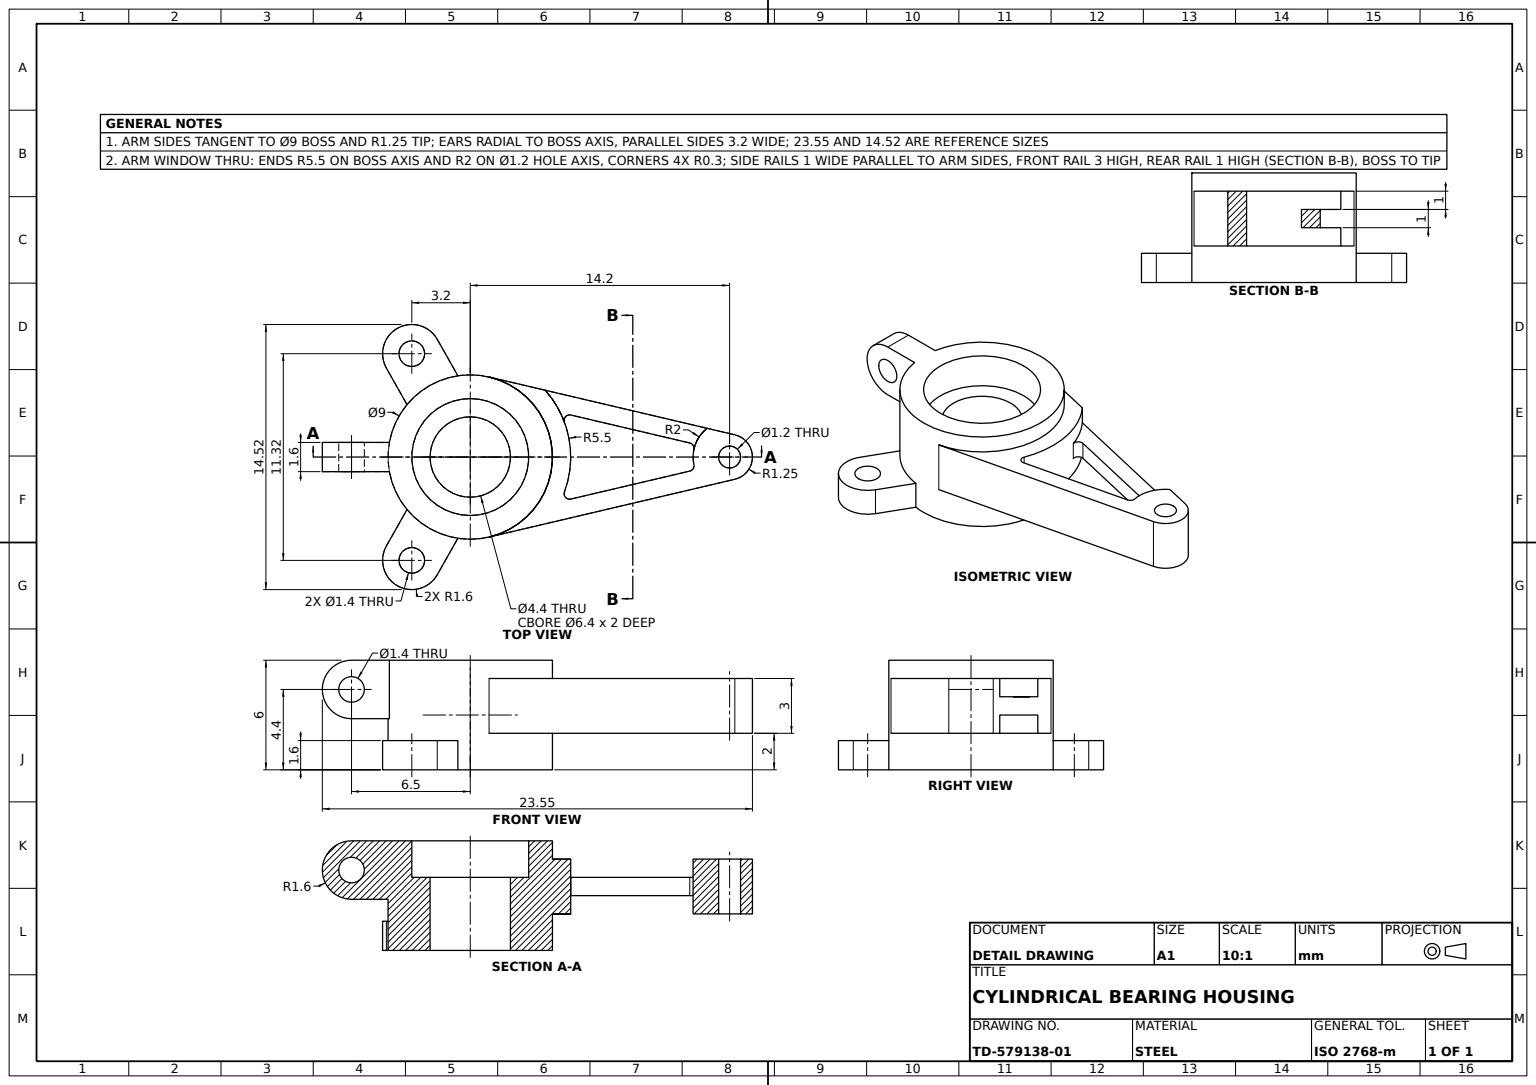
from build123d import *

# Parameters (mm, degrees)
HUB_PROFILE_SKETCH_R           = 4.5
HUB_CYLINDER_DEPTH             = 6
ARM_START                      = -4
ARM_DEPTH                      = 3
FLAT_EAR_PROFILE_SKETCH_R      = 0.7
FLAT_MOUNTING_EAR_DEPTH        = 1.6
UPRIGHT_EAR_PROFILE_SKETCH_R   = 0.7
UPRIGHT_MOUNTING_EAR_DEPTH     = 0.8
UPRIGHT_EAR_EXTENSION_SKETCH_W = 1.6
UPRIGHT_EAR_EXTENSION_SKETCH_H = 3.2
UPRIGHT_EAR_EXTENSION_DEPTH    = 0.8
HUB_BORE_CBORE_4_4_D           = 4.4
HUB_BORE_CBORE_4_4_DEPTH       = 100
HUB_BORE_CBORE_4_4_CBORE_D     = 6.4
HUB_BORE_CBORE_4_4_CBORE_DEPTH = 2
ARM_FRAME_CUT_DEPTH            = 18.786996987
ARM_FRAME_CUT_DEPTH_BACK       = 18.786996987
ARM_FRAME_CUT_SKETCH_R         = 0.6
ARM_START_2                    = -1
ARM_WINDOW_CUT_A_DEPTH         = 1
ARM_START_3                    = -3
ARM_WINDOW_CUT_B_DEPTH         = 1


with BuildPart() as part:
    # Hub Profile Sketch → Hub Cylinder (new body)
    with BuildSketch(Plane(origin=(0, 0, 0), x_dir=(1, 0, 0), z_dir=(0, 1, 0))):
        with Locations(Location((0, 0, 0), (0, 0, 270))):
            Circle(HUB_PROFILE_SKETCH_R)
    extrude(amount=HUB_CYLINDER_DEPTH)

    # Arm Profile Sketch → Arm (add)
    with BuildSketch(Plane(origin=(0, 6, 0), x_dir=(1, 0, 0), z_dir=(0, 1, 0)).offset(ARM_START)):
        with BuildLine():
            Line((1.029929577, 4.380553055), (14.486091549, 1.216820293))
            ThreePointArc((14.486091549, 1.216820293), (15.45, 0), (14.486091549, -1.216820293))
            Line((14.486091549, -1.216820293), (1.029929577, -4.380553055))
            ThreePointArc((1.029929577, -4.380553055), (4.5, 0), (1.029929577, 4.380553055))
        make_face()
    extrude(amount=ARM_DEPTH)

    # Flat Ear Profile Sketch → Flat Mounting Ear (add)
    # profile 1 of 2: a face of its own
    with BuildSketch(Plane.XZ):
        with BuildLine():
            Line((-0.677946652, 4.448638931), (-1.807326015, 6.445430372))
            ThreePointArc((-1.807326015, 6.445430372), (-3.987692308, 7.050412049), (-4.592673985, 4.870045756))
            Line((-4.592673985, 4.870045756), (-3.463294622, 2.873254315))
            ThreePointArc((-3.463294622, 2.873254315), (-2.215384615, 3.916895583), (-0.677946652, 4.448638931))
        make_face()
        with Locations(Location((-3.2, 5.657738064, 0), (0, 0, 270))):
            Circle(FLAT_EAR_PROFILE_SKETCH_R, mode=Mode.SUBTRACT)
    # profile 2 of 2: a face of its own
    with BuildSketch(Plane.XZ):
        with BuildLine():
            Line((-0.677946652, -4.448638931), (-1.807326015, -6.445430372))
            ThreePointArc((-1.807326015, -6.445430372), (-3.987692308, -7.050412049), (-4.592673985, -4.870045756))
            Line((-4.592673985, -4.870045756), (-3.463294622, -2.873254315))
            ThreePointArc((-3.463294622, -2.873254315), (-2.215384615, -3.916895583), (-0.677946652, -4.448638931))
        make_face()
        with Locations(Location((-3.2, -5.657738064, 0), (0, 0, 270))):
            Circle(FLAT_EAR_PROFILE_SKETCH_R, mode=Mode.SUBTRACT)
    extrude(amount=-FLAT_MOUNTING_EAR_DEPTH)



with BuildPart() as body_2:
    # Upright Ear Profile Sketch → Upright Mounting Ear (new, symmetric)
    with BuildSketch(Plane.XY):
        with BuildLine():
            Line((-4.5, 6), (-6.5, 6))
            ThreePointArc((-6.5, 6), (-8.1, 4.4), (-6.5, 2.8))
            Line((-6.5, 2.8), (-4.5, 2.8))
            Line((-4.5, 2.8), (-4.5, 6))
        make_face()
        with Locations((-6.5, 4.4)):
            Circle(UPRIGHT_EAR_PROFILE_SKETCH_R, mode=Mode.SUBTRACT)
    extrude(amount=UPRIGHT_MOUNTING_EAR_DEPTH, both=True)


with BuildPart() as part_1:
    add(part.part)

    add(body_2.part)  # Upright Ear Extension merges body 2
    # Upright Ear Extension Sketch → Upright Ear Extension (add, symmetric)
    with BuildSketch(Plane(origin=(-4.5, 0, 0), x_dir=(0, 0, -1), z_dir=(1, 0, 0))):
        with Locations((0, 4.4)):
            Rectangle(UPRIGHT_EAR_EXTENSION_SKETCH_W, UPRIGHT_EAR_EXTENSION_SKETCH_H)
    extrude(amount=UPRIGHT_EAR_EXTENSION_DEPTH, both=True)

    # Hub Bore CBore _4.4
    with Locations(Plane(origin=(0, 6, 0), x_dir=(1, 0, 0), z_dir=(0, 1, 0))):
        with Locations((0, 0)):
            CounterBoreHole(HUB_BORE_CBORE_4_4_D / 2, HUB_BORE_CBORE_4_4_CBORE_D / 2, HUB_BORE_CBORE_4_4_CBORE_DEPTH, depth=HUB_BORE_CBORE_4_4_DEPTH)

    # Arm Frame Cut Sketch → Arm Frame Cut (cut, two sides: drawn at the far end of the back side and taken through both)
    with BuildSketch(Plane(origin=(0, 5, 0), x_dir=(1, 0, 0), z_dir=(0, 1, 0)).offset(-ARM_FRAME_CUT_DEPTH_BACK)):
        with Locations(Location((14.2, 0, 0), (0, 0, 270))):
            Circle(ARM_FRAME_CUT_SKETCH_R)
        with BuildLine():
            Line((12.018798086, 0.769648107), (5.510009379, 2.299955792))
            ThreePointArc((5.510009379, 2.299955792), (5.216619254, 2.20665809), (5.159898403, 1.904061046))
            ThreePointArc((5.159898403, 1.904061046), (5.5, 0), (5.159898403, -1.904061046))
            ThreePointArc((5.159898403, -1.904061046), (5.216619254, -2.20665809), (5.510009379, -2.299955792))
            Line((5.510009379, -2.299955792), (12.018798086, -0.769648107))
            ThreePointArc((12.018798086, -0.769648107), (12.203456694, -0.638324285), (12.243596621, -0.415314119))
            ThreePointArc((12.243596621, -0.415314119), (12.2, 0), (12.243596621, 0.415314119))
            ThreePointArc((12.243596621, 0.415314119), (12.203456694, 0.638324285), (12.018798086, 0.769648107))
        make_face()
    extrude(amount=ARM_FRAME_CUT_DEPTH + ARM_FRAME_CUT_DEPTH_BACK, mode=Mode.SUBTRACT)

    # Arm Window Sketch → Arm Window Cut A (cut)
    with BuildSketch(Plane(origin=(0, 5, 0), x_dir=(1, 0, 0), z_dir=(0, 1, 0)).offset(ARM_START_2)):
        with BuildLine():
            Line((12.96628349, 1.574148524), (4.108268481, 3.656792323))
            ThreePointArc((4.108268481, 3.656792323), (4.716221589, 2.829709158), (5.159898403, 1.904061046))
            ThreePointArc((5.159898403, 1.904061046), (5.216619254, 2.20665809), (5.510009379, 2.299955792))
            Line((5.510009379, 2.299955792), (12.018798086, 0.769648107))
            ThreePointArc((12.018798086, 0.769648107), (12.203456694, 0.638324285), (12.243596621, 0.415314119))
            ThreePointArc((12.243596621, 0.415314119), (12.502961249, 1.058328625), (12.96628349, 1.574148524))
        make_face()
    extrude(amount=ARM_WINDOW_CUT_A_DEPTH, mode=Mode.SUBTRACT)

    # Sketch12_2 → Arm Window Cut B (cut)
    with BuildSketch(Plane(origin=(0, 5, 0), x_dir=(1, 0, 0), z_dir=(0, 1, 0)).offset(ARM_START_3)):
        with BuildLine():
            Line((12.96628349, 1.574148524), (4.108268481, 3.656792323))
            ThreePointArc((4.108268481, 3.656792323), (4.716221589, 2.829709158), (5.159898403, 1.904061046))
            ThreePointArc((5.159898403, 1.904061046), (5.216619254, 2.20665809), (5.510009379, 2.299955792))
            Line((5.510009379, 2.299955792), (12.018798086, 0.769648107))
            ThreePointArc((12.018798086, 0.769648107), (12.203456694, 0.638324285), (12.243596621, 0.415314119))
            ThreePointArc((12.243596621, 0.415314119), (12.502961249, 1.058328625), (12.96628349, 1.574148524))
        make_face()
    extrude(amount=ARM_WINDOW_CUT_B_DEPTH, mode=Mode.SUBTRACT)


solid = part_1.part
